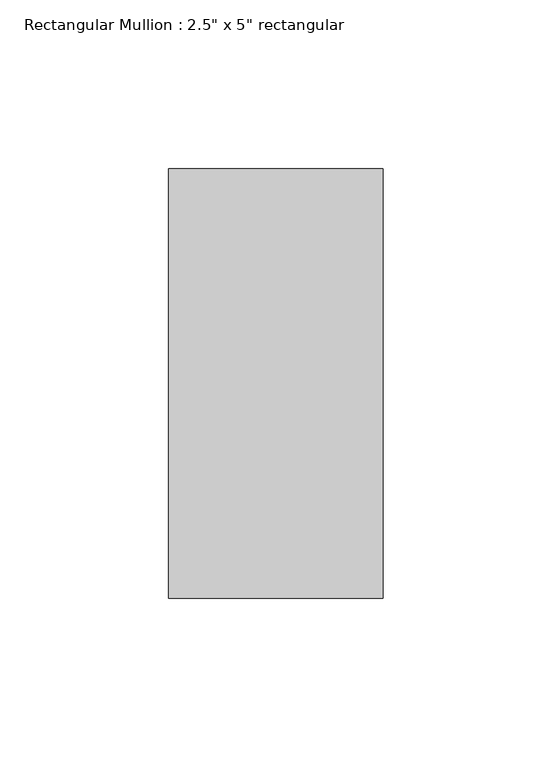
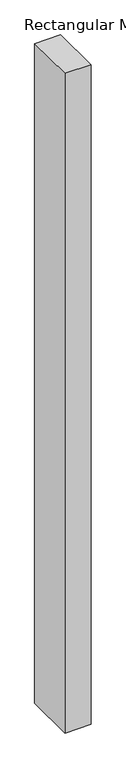
"""IFC4 building model written with IfcOpenShell, lengths in millimetres: member geometry."""

from ifc_helpers import new_model, si_unit, frame, origin, place, context, project, spatial, polyline, outline, extrude, source, transform, mapped, element, save


def member_4a676c08(model_context):
    return source(origin(), model_context, "Body", "SweptSolid", [
        extrude(outline(polyline([(31.75, 63.5), (31.75, -63.5), (-31.75, -63.5), (-31.75, 63.5), (31.75, 63.5)])), frame((0.0, 0.0, -1697.4525236), z_axis=(0.0, 0.0, 1.0), x_axis=(1.0, 0.0, 0.0)), (0.0, 0.0, 1.0), 1697.4525236),
    ])


if __name__ == "__main__":
    model = new_model("IFC4")
    model_context = context("Model", 3, world=origin())
    ifc_project = project(units=[si_unit("LENGTHUNIT", "METRE", prefix="MILLI")], contexts=[model_context])
    site = spatial("IfcSite", under=ifc_project)
    building = spatial("IfcBuilding", under=site)
    placement = place(None, origin())
    member_shape = member_4a676c08(model_context)
    element("IfcMember", 1, ObjectType="Rectangular Mullion : 2.5\" x 5\" rectangular", at=placement, inside=building, context=model_context, shape_type="MappedRepresentation", body=[
        mapped(member_shape, transform((0.0, 0.0, 0.0), x_axis=(1.0, 0.0, 0.0), y_axis=(0.0, 1.0, 0.0), z_axis=(0.0, 0.0, 1.0))),
    ])
    save(model, "model.ifc")

# Revit data of these elements
# Type "Rectangular Mullion : 2.5\" x 5\" rectangular"
#   built-in parameter 1007304 = 0.416667 (stored number, unit not read)
#   built-in parameter 1007301 = 0.104167 (stored number, unit not read)
#   built-in parameter 1007300 = 0.104167 (stored number, unit not read)
# Element 1 (IfcMember, "Rectangular Mullion : 2.5\" x 5\" rectangular")
#   Materials on its faces: "Aluminum"
# Materials
#   "Aluminum": class "Metal", colour RGB 247 247 247, transparency 0, Description = "Aluminum 6061", Cost = 0
